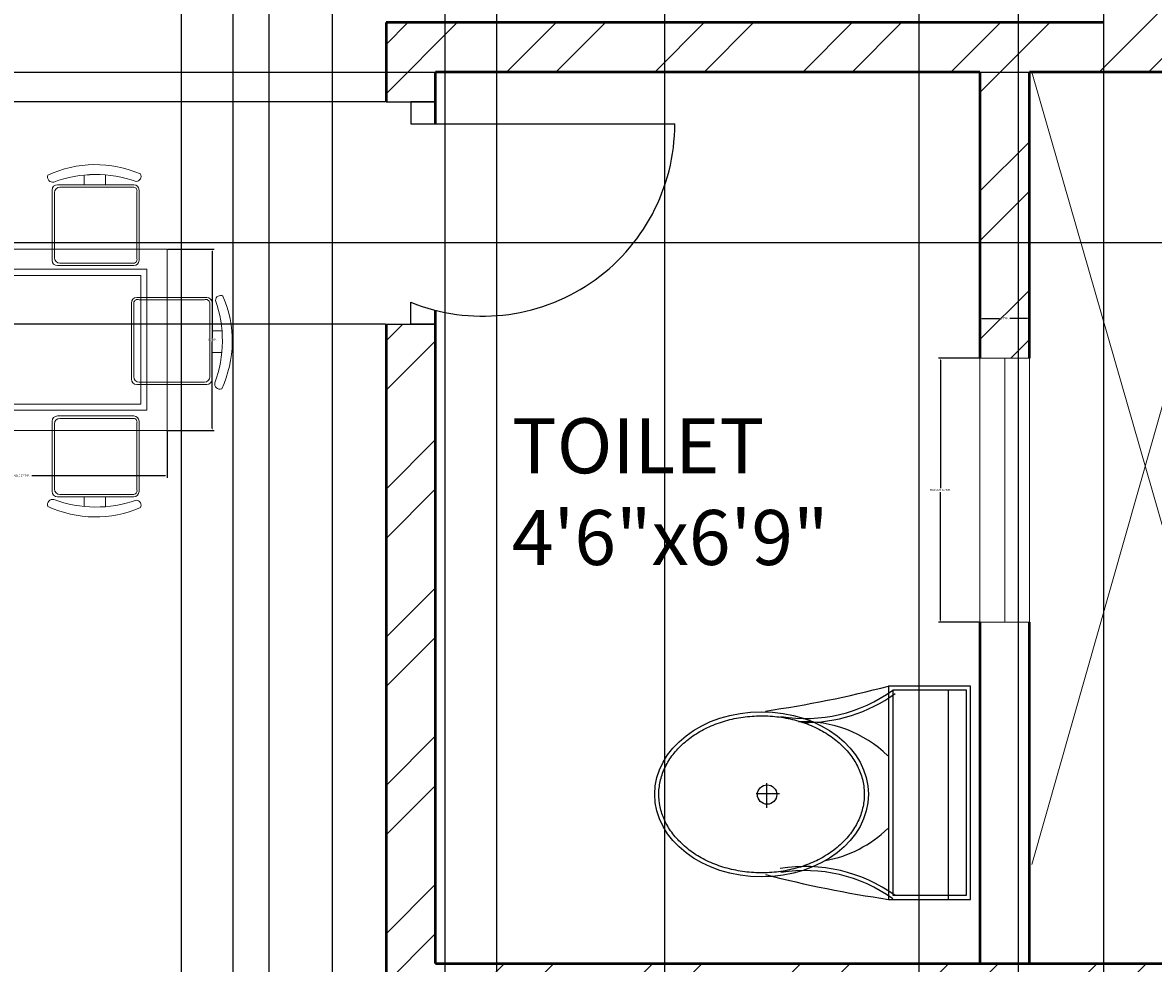
# Model space of a CAD drawing. Units: inches. Extents: x 1980 to 2738, y 1471 to 2568.
# Tile 6 of 22: x 2260 to 2363, y 1792 to 1878. Entities that reach past the tile are written whole.
import ezdxf

# ---------------------------------------------------------------- set-up
doc = ezdxf.new("R2010")
doc.units = ezdxf.units.IN
for name, color, linetype, lineweight in [('A-ANNO-DIMS', 2, 'Continuous', 18), ('A-AREA-IDEN', 7, 'Continuous', 18), ('A-DOOR', 31, 'Continuous', 25), ('A-FLOR-FIXT', 8, 'Continuous', 25), ('A-FLOR-OPEN', 8, 'Continuous', 18), ('A-FURN', 8, 'Continuous', 18), ('A-GLAZ', 141, 'Continuous', 18), ('A-WALL', 7, 'Continuous', 50)]:
    doc.layers.add(name, color=color, linetype=linetype, lineweight=lineweight)
doc.layers.add('A-WALL-PATT', color=9, linetype='Continuous', lineweight=13, true_color=0xd19cc7)
doc.styles.get("Standard").update_dxf_attribs({"font": 'arial.ttf'})
doc.dimstyles.get("Standard").update_dxf_attribs({"dimtxt": 0.18, "dimasz": 0.18, "dimexe": 0.18, "dimexo": 0.0625, "dimgap": 0.09, "dimtad": 0, "dimtih": 1, "dimtoh": 1, "dimdec": 4, "dimzin": 0, "dimdsep": 46, "dimtxsty": 'Standard', "dimcen": 0.09, "dimadec": 0, "dimazin": 0, "dimtfac": 1, "dimtdec": 4, "dimtofl": 0, "dimtmove": 0, "dimatfit": 3, "dimfxl": 1, "dimtolj": 1, "dimtzin": 0, "dimarcsym": 0})

# ---------------------------------------------------------------- blocks, each defined once
blk = doc.blocks.new('A$C31115884')
for p, q in [((283.1, 497.7), (223.4, 497.7)), ((257.5, 466.4), (257.5, 523.2)), ((0, 200), (0, 0)), ((520, 200), (0, 200)), ((520, 0), (520, 200)), ((10, 190), (10, 10)), ((510, 190), (10, 190)), ((510, 10), (510, 190)), ((510, 54.5), (0, 54.5)), ((10, 10), (510, 10)), ((0, 0), (520, 0))]:
    blk.add_line(p, q)
blk.add_circle((255.6, 496.4), 23.6)
for centre, radius, start, end in [((2777.7, -204.6), 2807, 165.4549, 171.7133), ((3237, 905), 2807, 188.2867, 194.5451), ((-294.5, 403.3), 364.7, 324.2091, 9.3499), ((-294.5, 403.3), 374.7, 324.2091, 9.3499), ((805.8, 403.3), 364.7, 170.6501, 215.7909), ((139.5, 406.2), 293.5, 315.8436, 2.6563), ((805.8, 403.3), 374.7, 179.2036, 215.7909), ((383.6, 406.2), 293.5, 190.2774, 224.1564)]:
    blk.add_arc(centre, radius, start, end)
blk.add_ellipse((256.2, 509.9), major_axis=(0, -260.7), ratio=0.772727)
blk.add_open_spline([(256.2, 259.2), (263.1, 259.2), (270, 259.7), (287.8, 262.3), (298.7, 265.1), (319.9, 273.1), (330.2, 278.4), (350.1, 291.1), (359.7, 298.7), (377.7, 315.9), (386.2, 325.5), (401.7, 346.6), (408.8, 358.1), (421.3, 382.5), (426.8, 395.5), (435.9, 422.4), (439.5, 436.4), (444.8, 465.1), (446.5, 479.7), (447.9, 509.2), (447.6, 524), (445, 553.3), (442.7, 567.8), (436.3, 596), (432.1, 609.7), (421.9, 636), (416, 648.6), (402.5, 672.1), (395, 683), (378.6, 703), (369.8, 712.1), (351.1, 728), (341.3, 734.8), (320.9, 746.2), (310.4, 750.7), (288.9, 757.3), (278, 759.4), (256, 761), (245, 760.6), (223.1, 757.2), (212.3, 754.3), (191.1, 746.1), (180.8, 740.7), (160.9, 727.8), (151.4, 720.1), (133.5, 702.7), (125.1, 693), (109.6, 671.7), (102.6, 660.2), (90.2, 635.7), (84.9, 622.7), (76, 595.6), (72.4, 581.6), (67.2, 552.9), (65.6, 538.2), (64.4, 508.8), (64.8, 494), (67.5, 464.7), (69.9, 450.2), (76.6, 422), (80.8, 408.3), (91.1, 382.2), (97.2, 369.7), (110.8, 346.3), (118.4, 335.4), (134.8, 315.6), (143.7, 306.7), (162.4, 290.9), (172.3, 284.2), (192.8, 273), (203.3, 268.6), (224.8, 262.2), (235.8, 260.2), (249.9, 259.3), (253, 259.2), (256.2, 259.2)], degree=3, knots=[0, 0, 0, 0, 0.110105, 0.110105, 0.285049, 0.285049, 0.459994, 0.459994, 0.634938, 0.634938, 0.809882, 0.809882, 0.984827, 0.984827, 1.159771, 1.159771, 1.334715, 1.334715, 1.50966, 1.50966, 1.684604, 1.684604, 1.859549, 1.859549, 2.034493, 2.034493, 2.209437, 2.209437, 2.384382, 2.384382, 2.559326, 2.559326, 2.73427, 2.73427, 2.909215, 2.909215, 3.084159, 3.084159, 3.259103, 3.259103, 3.434048, 3.434048, 3.608992, 3.608992, 3.783936, 3.783936, 3.958881, 3.958881, 4.133825, 4.133825, 4.30877, 4.30877, 4.483714, 4.483714, 4.658658, 4.658658, 4.833603, 4.833603, 5.008547, 5.008547, 5.183491, 5.183491, 5.358436, 5.358436, 5.53338, 5.53338, 5.708324, 5.708324, 5.883269, 5.883269, 6.058213, 6.058213, 6.233158, 6.233158, 6.283185, 6.283185, 6.283185, 6.283185])
blk = doc.blocks.new('TABLE-DINING-RECT')
for points in [[(0, 16.47), (27.45, 16.47), (27.45, 0), (0, 0)], [(0, 16.47), (27.45, 16.47), (27.45, 0), (0, 0)], [(1.83, 14.64), (25.62, 14.64), (25.62, 1.83), (1.83, 1.83)], [(1.83, 14.64), (25.62, 14.64), (25.62, 1.83), (1.83, 1.83)], [(2.38, 14.09), (25.07, 14.09), (25.07, 2.38), (2.38, 2.38)], [(2.38, 14.09), (25.07, 14.09), (25.07, 2.38), (2.38, 2.38)]]:
    blk.add_lwpolyline(points, close=True)
blk = doc.blocks.new('WIN-24IN-PARTITION')
for p, q in [((0, 24), (4.5, 24)), ((0, 24), (0, 0)), ((4.5, 24), (2.25, 24)), ((2.25, 24), (2.25, 0)), ((4.5, 24), (4.5, 0)), ((2.25, 0), (0, 0)), ((0, 0), (4.5, 0))]:
    blk.add_line(p, q)
blk = doc.blocks.new('SHAFT-OPENING-MARK')
for p, q in [((20.51, 72), (0, 0)), ((0, 72), (20.71, 0.06))]:
    blk.add_line(p, q)
blk = doc.blocks.new('*D21')
at = {"layer": 'A-ANNO-DIMS', "color": 0, "lineweight": -2, "transparency": 16777216}
for p, q in [((2245.93, 1840.58), (2245.93, 1836.35)), ((2273.38, 1840.58), (2273.38, 1836.35)), ((2246.11, 1836.53), (2258.22, 1836.53)), ((2273.2, 1836.53), (2261.09, 1836.53))]:
    blk.add_line(p, q, dxfattribs=at)
at = {"layer": 'A-ANNO-DIMS', "color": 0, "transparency": 16777216}
for points in [[(2246.11, 1836.56), (2246.11, 1836.5), (2245.93, 1836.53)], [(2273.2, 1836.56), (2273.2, 1836.5), (2273.38, 1836.53)]]:
    blk.add_solid(points, dxfattribs=at)
at = {"layer": 'Defpoints', "color": 0, "transparency": 16777216}
for p in [(2245.93, 1840.64), (2273.38, 1840.64), (2273.38, 1836.53)]:
    blk.add_point(p, dxfattribs=at)
at = {"layer": 'A-ANNO-DIMS', "color": 0, "transparency": 16777216, "insert": (2259.65, 1836.53), "char_height": 0.18, "attachment_point": 5}
blk.add_mtext('\\A1;DINING TABLE 27 TYP.', dxfattribs=at)
blk = doc.blocks.new('*D22')
at = {"layer": 'A-ANNO-DIMS', "color": 0, "lineweight": -2, "transparency": 16777216}
for p, q in [((2273.44, 1857.11), (2277.67, 1857.11)), ((2277.49, 1856.93), (2277.49, 1849.06)), ((2277.49, 1840.82), (2277.49, 1848.7)), ((2273.44, 1840.64), (2277.67, 1840.64))]:
    blk.add_line(p, q, dxfattribs=at)
at = {"layer": 'A-ANNO-DIMS', "color": 0, "transparency": 16777216}
for points in [[(2277.46, 1856.93), (2277.52, 1856.93), (2277.49, 1857.11)], [(2277.46, 1840.82), (2277.52, 1840.82), (2277.49, 1840.64)]]:
    blk.add_solid(points, dxfattribs=at)
at = {"layer": 'Defpoints', "color": 0, "transparency": 16777216}
for p in [(2273.38, 1857.11), (2277.49, 1857.11), (2273.38, 1840.64)]:
    blk.add_point(p, dxfattribs=at)
at = {"layer": 'A-ANNO-DIMS', "color": 0, "transparency": 16777216, "insert": (2277.49, 1848.88), "char_height": 0.18, "attachment_point": 5}
blk.add_mtext('\\A1;16 TYP.', dxfattribs=at)
blk = doc.blocks.new('*D25')
at = {"layer": 'A-ANNO-DIMS', "color": 0, "lineweight": -2, "transparency": 16777216}
for p, q in [((2347.25, 1847.22), (2343.53, 1847.22)), ((2343.71, 1847.04), (2343.71, 1835.4)), ((2343.71, 1823.4), (2343.71, 1835.04)), ((2347.25, 1823.22), (2343.53, 1823.22))]:
    blk.add_line(p, q, dxfattribs=at)
at = {"layer": 'A-ANNO-DIMS', "color": 0, "transparency": 16777216}
for points in [[(2343.68, 1847.04), (2343.74, 1847.04), (2343.71, 1847.22)], [(2343.68, 1823.4), (2343.74, 1823.4), (2343.71, 1823.22)]]:
    blk.add_solid(points, dxfattribs=at)
at = {"layer": 'Defpoints', "color": 0, "transparency": 16777216}
for p in [(2343.71, 1847.22), (2347.31, 1847.22), (2347.31, 1823.22)]:
    blk.add_point(p, dxfattribs=at)
at = {"layer": 'A-ANNO-DIMS', "color": 0, "transparency": 16777216, "insert": (2343.71, 1835.22), "char_height": 0.18, "attachment_point": 5}
blk.add_mtext('\\A1;WINDOW 24 TYP.', dxfattribs=at)
blk = doc.blocks.new('*D26')
at = {"layer": 'A-ANNO-DIMS', "color": 0, "lineweight": -2, "transparency": 16777216}
for p, q in [((2347.31, 1847.28), (2347.31, 1851)), ((2347.49, 1850.82), (2349.1, 1850.82)), ((2351.63, 1850.82), (2350.02, 1850.82)), ((2351.81, 1847.28), (2351.81, 1851))]:
    blk.add_line(p, q, dxfattribs=at)
at = {"layer": 'A-ANNO-DIMS', "color": 0, "transparency": 16777216}
for points in [[(2347.49, 1850.85), (2347.49, 1850.79), (2347.31, 1850.82)], [(2351.63, 1850.85), (2351.63, 1850.79), (2351.81, 1850.82)]]:
    blk.add_solid(points, dxfattribs=at)
at = {"layer": 'Defpoints', "color": 0, "transparency": 16777216}
for p in [(2351.81, 1850.82), (2347.31, 1847.22), (2351.81, 1847.22)]:
    blk.add_point(p, dxfattribs=at)
at = {"layer": 'A-ANNO-DIMS', "color": 0, "transparency": 16777216, "insert": (2349.56, 1850.82), "char_height": 0.18, "attachment_point": 5}
blk.add_mtext('\\A1;5 TYP.', dxfattribs=at)
blk = doc.blocks.new('*D40')
at = {"layer": 'A-ANNO-DIMS', "color": 0, "lineweight": -2, "transparency": 16777216}
for p, q in [((2218.65, 2053.14), (2218.65, 1533.71)), ((2298.65, 2053.14), (2298.65, 1533.71)), ((2218.83, 1533.89), (2258.43, 1533.89)), ((2298.47, 1533.89), (2258.87, 1533.89))]:
    blk.add_line(p, q, dxfattribs=at)
at = {"layer": 'A-ANNO-DIMS', "color": 0, "transparency": 16777216}
for points in [[(2218.83, 1533.92), (2218.83, 1533.86), (2218.65, 1533.89)], [(2298.47, 1533.92), (2298.47, 1533.86), (2298.65, 1533.89)]]:
    blk.add_solid(points, dxfattribs=at)
at = {"layer": 'Defpoints', "color": 0, "transparency": 16777216}
for p in [(2218.65, 2053.21), (2298.65, 2053.21), (2298.65, 1533.89)]:
    blk.add_point(p, dxfattribs=at)
at = {"layer": 'A-ANNO-DIMS', "color": 0, "transparency": 16777216, "insert": (2258.65, 1533.89), "char_height": 0.18, "attachment_point": 5}
blk.add_mtext('\\A1;80', dxfattribs=at)
blk = doc.blocks.new('*D41')
at = {"layer": 'A-ANNO-DIMS', "color": 0, "lineweight": -2, "transparency": 16777216}
for p, q in [((2298.65, 2095.14), (2298.65, 1533.71)), ((2515.4, 2095.14), (2515.4, 1533.71)), ((2298.83, 1533.89), (2406.56, 1533.89)), ((2515.22, 1533.89), (2407.49, 1533.89))]:
    blk.add_line(p, q, dxfattribs=at)
at = {"layer": 'A-ANNO-DIMS', "color": 0, "transparency": 16777216}
for points in [[(2298.83, 1533.92), (2298.83, 1533.86), (2298.65, 1533.89)], [(2515.22, 1533.92), (2515.22, 1533.86), (2515.4, 1533.89)]]:
    blk.add_solid(points, dxfattribs=at)
at = {"layer": 'Defpoints', "color": 0, "transparency": 16777216}
for p in [(2298.65, 2095.21), (2515.4, 2095.21), (2515.4, 1533.89)]:
    blk.add_point(p, dxfattribs=at)
at = {"layer": 'A-ANNO-DIMS', "color": 0, "transparency": 16777216, "insert": (2407.03, 1533.89), "char_height": 0.18, "attachment_point": 5}
blk.add_mtext('\\A1;216.75', dxfattribs=at)
blk = doc.blocks.new('*D45')
at = {"layer": 'A-ANNO-DIMS', "color": 0, "lineweight": -2, "transparency": 16777216}
for p, q in [((2255.99, 1694.77), (2255.99, 2507.54)), ((2256.17, 2507.36), (2267.22, 2507.36)), ((2279.21, 2507.36), (2268.15, 2507.36)), ((2279.39, 1694.77), (2279.39, 2507.54))]:
    blk.add_line(p, q, dxfattribs=at)
at = {"layer": 'A-ANNO-DIMS', "color": 0, "transparency": 16777216}
for points in [[(2256.17, 2507.39), (2256.17, 2507.33), (2255.99, 2507.36)], [(2279.21, 2507.39), (2279.21, 2507.33), (2279.39, 2507.36)]]:
    blk.add_solid(points, dxfattribs=at)
at = {"layer": 'Defpoints', "color": 0, "transparency": 16777216}
for p in [(2279.39, 2507.36), (2255.99, 1694.71), (2279.39, 1694.71)]:
    blk.add_point(p, dxfattribs=at)
at = {"layer": 'A-ANNO-DIMS', "color": 0, "transparency": 16777216, "insert": (2267.69, 2507.36), "char_height": 0.18, "attachment_point": 5}
blk.add_mtext('\\A1;23.407', dxfattribs=at)
blk = doc.blocks.new('*D50')
at = {"layer": 'A-ANNO-DIMS', "color": 0, "lineweight": -2, "transparency": 16777216}
for p, q in [((2288.43, 1708.09), (2288.43, 2507.54)), ((2288.61, 2507.36), (2314.71, 2507.36)), ((2341.6, 2507.36), (2315.5, 2507.36)), ((2341.78, 1708.09), (2341.78, 2507.54))]:
    blk.add_line(p, q, dxfattribs=at)
at = {"layer": 'A-ANNO-DIMS', "color": 0, "transparency": 16777216}
for points in [[(2288.61, 2507.39), (2288.61, 2507.33), (2288.43, 2507.36)], [(2341.6, 2507.39), (2341.6, 2507.33), (2341.78, 2507.36)]]:
    blk.add_solid(points, dxfattribs=at)
at = {"layer": 'Defpoints', "color": 0, "transparency": 16777216}
for p in [(2341.78, 2507.36), (2288.43, 1708.03), (2341.78, 1708.03)]:
    blk.add_point(p, dxfattribs=at)
at = {"layer": 'A-ANNO-DIMS', "color": 0, "transparency": 16777216, "insert": (2315.11, 2507.36), "char_height": 0.18, "attachment_point": 5}
blk.add_mtext('\\A1;53.34', dxfattribs=at)
blk = doc.blocks.new('*D51')
at = {"layer": 'A-ANNO-DIMS', "color": 0, "lineweight": -2, "transparency": 16777216}
for p, q in [((2341.78, 1708.09), (2341.78, 2507.54)), ((2341.96, 2507.36), (2349.72, 2507.36)), ((2358.4, 2507.36), (2350.63, 2507.36)), ((2358.58, 1694.77), (2358.58, 2507.54))]:
    blk.add_line(p, q, dxfattribs=at)
at = {"layer": 'A-ANNO-DIMS', "color": 0, "transparency": 16777216}
for points in [[(2341.96, 2507.39), (2341.96, 2507.33), (2341.78, 2507.36)], [(2358.4, 2507.39), (2358.4, 2507.33), (2358.58, 2507.36)]]:
    blk.add_solid(points, dxfattribs=at)
at = {"layer": 'Defpoints', "color": 0, "transparency": 16777216}
for p in [(2358.58, 2507.36), (2341.78, 1708.03), (2358.58, 1694.71)]:
    blk.add_point(p, dxfattribs=at)
at = {"layer": 'A-ANNO-DIMS', "color": 0, "transparency": 16777216, "insert": (2350.18, 2507.36), "char_height": 0.18, "attachment_point": 5}
blk.add_mtext('\\A1;16.807', dxfattribs=at)
blk = doc.blocks.new('*D53')
at = {"layer": 'A-ANNO-DIMS', "color": 0, "lineweight": -2, "transparency": 16777216}
for p, q in [((2318.63, 2002.14), (2318.63, 1533.71)), ((2350.79, 2002.14), (2350.79, 1533.71)), ((2318.81, 1533.89), (2334.25, 1533.89)), ((2350.61, 1533.89), (2335.18, 1533.89))]:
    blk.add_line(p, q, dxfattribs=at)
at = {"layer": 'A-ANNO-DIMS', "color": 0, "transparency": 16777216}
for points in [[(2318.81, 1533.92), (2318.81, 1533.86), (2318.63, 1533.89)], [(2350.61, 1533.92), (2350.61, 1533.86), (2350.79, 1533.89)]]:
    blk.add_solid(points, dxfattribs=at)
at = {"layer": 'Defpoints', "color": 0, "transparency": 16777216}
for p in [(2318.63, 2002.21), (2350.79, 2002.21), (2350.79, 1533.89)]:
    blk.add_point(p, dxfattribs=at)
at = {"layer": 'A-ANNO-DIMS', "color": 0, "transparency": 16777216, "insert": (2334.71, 1533.89), "char_height": 0.18, "attachment_point": 5}
blk.add_mtext('\\A1;32.155', dxfattribs=at)
blk = doc.blocks.new('*D61')
at = {"layer": 'A-ANNO-DIMS', "color": 0, "lineweight": -2, "transparency": 16777216}
for p, q in [((2114.15, 1873.21), (2689.91, 1873.21)), ((2689.73, 1873.03), (2689.73, 1865.65)), ((2689.73, 1857.91), (2689.73, 1865.29)), ((2114.15, 1857.73), (2689.91, 1857.73))]:
    blk.add_line(p, q, dxfattribs=at)
at = {"layer": 'A-ANNO-DIMS', "color": 0, "transparency": 16777216}
for points in [[(2689.7, 1873.03), (2689.76, 1873.03), (2689.73, 1873.21)], [(2689.7, 1857.91), (2689.76, 1857.91), (2689.73, 1857.73)]]:
    blk.add_solid(points, dxfattribs=at)
at = {"layer": 'Defpoints', "color": 0, "transparency": 16777216}
for p in [(2114.08, 1873.21), (2689.73, 1873.21), (2114.08, 1857.73)]:
    blk.add_point(p, dxfattribs=at)
at = {"layer": 'A-ANNO-DIMS', "color": 0, "transparency": 16777216, "insert": (2689.73, 1865.47), "char_height": 0.18, "attachment_point": 5}
blk.add_mtext('\\A1;15.48', dxfattribs=at)
blk = doc.blocks.new('*D64')
at = {"layer": 'A-ANNO-DIMS', "color": 0, "lineweight": -2, "transparency": 16777216}
for p, q in [((2303.33, 2002.14), (2303.33, 1533.71)), ((2318.63, 2002.14), (2318.63, 1533.71)), ((2303.51, 1533.89), (2310.67, 1533.89)), ((2318.45, 1533.89), (2311.3, 1533.89))]:
    blk.add_line(p, q, dxfattribs=at)
at = {"layer": 'A-ANNO-DIMS', "color": 0, "transparency": 16777216}
for points in [[(2303.51, 1533.92), (2303.51, 1533.86), (2303.33, 1533.89)], [(2318.45, 1533.92), (2318.45, 1533.86), (2318.63, 1533.89)]]:
    blk.add_solid(points, dxfattribs=at)
at = {"layer": 'Defpoints', "color": 0, "transparency": 16777216}
for p in [(2303.33, 2002.21), (2318.63, 2002.21), (2318.63, 1533.89)]:
    blk.add_point(p, dxfattribs=at)
at = {"layer": 'A-ANNO-DIMS', "color": 0, "transparency": 16777216, "insert": (2310.98, 1533.89), "char_height": 0.18, "attachment_point": 5}
blk.add_mtext('\\A1;15.3', dxfattribs=at)
blk = doc.blocks.new('*D65')
at = {"layer": 'A-ANNO-DIMS', "color": 0, "lineweight": -2, "transparency": 16777216}
for p, q in [((2293.25, 1870.5), (2036.25, 1870.5)), ((2036.43, 1870.32), (2036.43, 1860.58)), ((2036.43, 1850.47), (2036.43, 1860.21)), ((2293.25, 1850.29), (2036.25, 1850.29))]:
    blk.add_line(p, q, dxfattribs=at)
at = {"layer": 'A-ANNO-DIMS', "color": 0, "transparency": 16777216}
for points in [[(2036.4, 1870.32), (2036.46, 1870.32), (2036.43, 1870.5)], [(2036.4, 1850.47), (2036.46, 1850.47), (2036.43, 1850.29)]]:
    blk.add_solid(points, dxfattribs=at)
at = {"layer": 'Defpoints', "color": 0, "transparency": 16777216}
for p in [(2036.43, 1870.5), (2293.31, 1870.5), (2293.31, 1850.29)]:
    blk.add_point(p, dxfattribs=at)
at = {"layer": 'A-ANNO-DIMS', "color": 0, "transparency": 16777216, "insert": (2036.43, 1860.4), "char_height": 0.18, "attachment_point": 5}
blk.add_mtext('\\A1;20.204', dxfattribs=at)
blk = doc.blocks.new('*D66')
at = {"layer": 'A-ANNO-DIMS', "color": 0, "lineweight": -2, "transparency": 16777216}
for p, q in [((2274.65, 2095.14), (2274.65, 1533.71)), ((2282.65, 2095.14), (2282.65, 1533.71)), ((2274.83, 1533.89), (2278.5, 1533.89)), ((2282.47, 1533.89), (2278.8, 1533.89))]:
    blk.add_line(p, q, dxfattribs=at)
at = {"layer": 'A-ANNO-DIMS', "color": 0, "transparency": 16777216}
for points in [[(2274.83, 1533.92), (2274.83, 1533.86), (2274.65, 1533.89)], [(2282.47, 1533.92), (2282.47, 1533.86), (2282.65, 1533.89)]]:
    blk.add_solid(points, dxfattribs=at)
at = {"layer": 'Defpoints', "color": 0, "transparency": 16777216}
for p in [(2274.65, 2095.21), (2282.65, 2095.21), (2282.65, 1533.89)]:
    blk.add_point(p, dxfattribs=at)
at = {"layer": 'A-ANNO-DIMS', "color": 0, "transparency": 16777216, "insert": (2278.65, 1533.89), "char_height": 0.18, "attachment_point": 5}
blk.add_mtext('\\A1;8', dxfattribs=at)

msp = doc.modelspace()

# ---------------------------------------------------------------- hatches: boundary and pattern name
at = {"layer": 'A-WALL-PATT'}
h = msp.add_hatch(dxfattribs=at)
h.set_pattern_fill('ANSI32', color=256)
h.paths.add_polyline_path([(2257.5661, 2416.2064), (2257.5661, 2420.7064), (2250.5833, 2420.7064), (2250.5833, 2462.7064), (2246.0833, 2462.7064), (2246.0833, 2420.7064), (2237.0791, 2420.7064), (2237.0791, 2411.7064), (2246.0833, 2411.7064), (2246.0833, 2291.7064), (2242.6109, 2291.7064), (2242.6109, 2287.2064), (2246.0833, 2287.2064), (2250.5833, 2287.2064), (2250.5833, 2291.7064), (2250.5833, 2411.7064), (2257.5661, 2411.7064)])
h.paths.add_polyline_path([(2387.0396, 2416.2064), (2387.0396, 2420.7064), (2367.5833, 2420.7064), (2367.5833, 2462.7064), (2358.5833, 2462.7064), (2358.5833, 2420.7064), (2329.3087, 2420.7064), (2329.3087, 2411.7064), (2358.5833, 2411.7064), (2358.5833, 2321.7275), (2358.5833, 2309.7064), (2347.3089, 2309.7064), (2293.3089, 2309.7064), (2293.3089, 2259.0771), (2297.8089, 2259.0771), (2297.8089, 2305.2064), (2347.3089, 2305.2064), (2347.3089, 2284.7412), (2351.8089, 2284.7412), (2351.8089, 2305.2064), (2372.3188, 2305.2064), (2372.3761, 2284.3899), (2377.0295, 2284.3899), (2377.0295, 2299.3058), (2377.0295, 2305.2064), (2426.5295, 2305.2064), (2426.5295, 2257.5573), (2431.0295, 2257.5573), (2431.0295, 2309.7064), (2377.0295, 2309.7064), (2367.5833, 2309.7064), (2367.5833, 2321.7275), (2367.5833, 2411.7064), (2387.0396, 2411.7064)])
h.paths.add_polyline_path([(2448.5267, 2416.2064), (2448.5267, 2420.7064), (2423.0396, 2420.7064), (2423.0396, 2411.7064), (2448.5267, 2411.7064)])
h.paths.add_polyline_path([(2130.9128, 2416.2064), (2130.9128, 2420.7064), (2105.0833, 2420.7064), (2105.0833, 2386.6942), (2114.0833, 2386.6942), (2114.0833, 2411.7064), (2130.9128, 2411.7064)])
h.paths.add_polyline_path([(2212.9478, 2420.7064), (2190.9128, 2420.7064), (2190.9128, 2411.7064), (2212.9478, 2411.7064), (2212.9478, 2416.2064)])
h.paths.add_polyline_path([(2114.0833, 2326.6942), (2105.0833, 2326.6942), (2105.0833, 2291.7064), (2081.0833, 2291.7064), (2081.0833, 2287.2064), (2105.0833, 2287.2064), (2105.0833, 2276.1935), (2114.0833, 2276.1935), (2114.0833, 2287.2064), (2166.3825, 2287.2064), (2166.3825, 2289.4564), (2166.3825, 2291.7064), (2114.0833, 2291.7064)])
h.paths.add_polyline_path([(2114.0833, 2252.1935), (2105.0833, 2252.1935), (2105.0833, 2233.2064), (2081.0833, 2233.2064), (2081.0833, 2228.7064), (2105.0833, 2228.7064), (2105.0833, 2213.4478), (2114.0833, 2213.4478), (2114.0833, 2228.7064), (2195.0833, 2228.7064), (2199.5833, 2228.7064), (2208.4455, 2228.7064), (2208.4455, 2230.9564), (2208.4455, 2233.2064), (2199.5833, 2233.2064), (2199.5833, 2287.2064), (2206.8904, 2287.2064), (2206.8904, 2289.4564), (2206.8904, 2291.7064), (2189.446, 2291.7064), (2189.446, 2289.4564), (2189.446, 2287.2064), (2195.0833, 2287.2064), (2195.0833, 2233.2064), (2114.0833, 2233.2064)])
h.paths.add_polyline_path([(2114.0833, 2153.4478), (2109.5833, 2153.4478), (2105.0833, 2153.4478), (2105.0833, 2135.2374), (2114.0833, 2135.2374)], flags=17)
h.paths.add_polyline_path([(2135.9619, 2095.4081), (2140.1805, 2095.4081), (2140.1805, 2104.2064), (2114.0833, 2104.2064), (2114.0833, 2110.3997), (2109.5833, 2110.3997), (2105.0833, 2110.3997), (2105.0833, 2104.2064), (2081.0833, 2104.2064), (2081.0833, 2099.7064), (2105.0833, 2099.7064), (2127.5416, 2099.8532), (2127.5416, 2056.9393), (2136.2133, 2056.9393)], flags=17)
h.paths.add_polyline_path([(2255.4895, 2104.2064), (2250.5833, 2104.2064), (2250.5833, 2233.2064), (2246.0833, 2233.2064), (2242.4941, 2233.2064), (2242.4941, 2228.7064), (2246.0833, 2228.7064), (2246.0833, 2104.2064), (2163.6825, 2104.2064), (2163.6825, 2099.8072), (2163.6825, 2095.4081), (2191.4325, 2095.4081), (2191.4325, 2011.2064), (2186.0833, 2011.2064), (2136.5143, 2010.8824), (2136.3702, 2032.9403), (2131.9559, 2032.9115), (2127.5416, 2032.8826), (2127.5416, 2006.7064), (2105.0833, 2006.7064), (2081.0833, 2006.7064), (2081.0833, 2002.2064), (2105.0833, 2002.2064), (2105.0833, 1995.9329), (2114.0833, 1995.9329), (2114.0833, 2002.2064), (2246.0833, 2002.2064), (2246.0833, 1877.7064), (2242.1358, 1877.7064), (2242.1358, 1873.2064), (2250.5833, 1873.2064), (2250.5833, 2002.2064), (2255.3335, 2002.2064), (2255.3335, 2011.2064), (2195.9325, 2011.2064), (2195.9325, 2095.2064), (2255.4895, 2095.2064), (2255.4895, 2099.5471)])
h.paths.add_polyline_path([(2199.5833, 1873.2064), (2209.827, 1873.2064), (2209.827, 1875.4564), (2209.827, 1877.7064), (2114.0833, 1877.7064), (2114.0833, 1890.0968), (2105.0833, 1890.0968), (2105.0833, 1877.7064), (2081.0833, 1877.7064), (2081.0833, 1873.2064), (2105.0833, 1873.2064), (2105.0833, 1857.7279), (2114.0833, 1857.7279), (2114.0833, 1873.2064), (2195.0833, 1873.2064), (2195.0833, 1819.2064), (2190.298, 1819.2064), (2190.298, 1814.7064), (2209.8976, 1814.7064), (2209.8976, 1816.9564), (2209.8976, 1819.2064), (2199.5833, 1819.2064)])
h.paths.add_polyline_path([(2114.0833, 1814.7064), (2166.2538, 1814.7064), (2166.2538, 1816.9564), (2166.2538, 1819.2064), (2114.0833, 1819.2064), (2114.0833, 1833.7279), (2109.5833, 1833.7279), (2105.0833, 1833.7279), (2105.0833, 1819.2064), (2081.0833, 1819.2064), (2081.0833, 1814.7064), (2105.0833, 1814.7064), (2105.0833, 1782.5516), (2114.0833, 1782.5516)])
h.paths.add_polyline_path([(2114.0833, 1722.5516), (2109.5833, 1722.5516), (2105.0833, 1722.5516), (2105.0833, 1685.7064), (2124.5104, 1685.7064), (2124.5104, 1690.2064), (2124.5104, 1694.7064), (2114.0833, 1694.7064)])
h.paths.add_polyline_path([(2218.8787, 1694.7064), (2184.5104, 1694.7064), (2184.5104, 1685.7064), (2218.8787, 1685.7064), (2218.8787, 1690.2064)])
h.paths.add_polyline_path([(2250.5833, 1819.2064), (2242.6431, 1819.2064), (2242.6431, 1816.9564), (2242.6431, 1814.7064), (2246.0833, 1814.7064), (2246.0833, 1694.7064), (2240.4035, 1694.7064), (2240.4035, 1690.2064), (2240.4035, 1685.7064), (2246.0833, 1685.7064), (2246.0833, 1643.7064), (2250.5833, 1643.7064), (2250.5833, 1685.7064), (2255.9859, 1685.7064), (2255.9859, 1690.2064), (2255.9859, 1694.7064), (2250.5833, 1694.7064)])
h.paths.add_polyline_path([(2297.4764, 1694.7064), (2279.3934, 1694.7064), (2279.3934, 1690.2064), (2279.3934, 1685.7064), (2297.4764, 1685.7064), (2297.4764, 1690.2064)])
h.paths.add_polyline_path([(2377.1596, 1694.7064), (2367.5833, 1694.7064), (2367.5833, 1787.7064), (2431.0295, 1787.7064), (2431.0295, 1792.2064), (2431.0295, 1849.4149), (2428.7795, 1849.4149), (2426.5295, 1849.4149), (2426.5295, 1792.2064), (2421.5833, 1792.2064), (2367.5833, 1792.2064), (2297.8089, 1792.2064), (2297.8089, 1850.2946), (2295.5589, 1850.2946), (2293.3089, 1850.2946), (2293.3089, 1792.2064), (2293.3089, 1787.7064), (2297.8089, 1787.7064), (2358.5833, 1787.7064), (2358.5833, 1694.7064), (2333.4764, 1694.7064), (2333.4764, 1685.7064), (2358.5833, 1685.7064), (2358.5833, 1643.7064), (2367.5833, 1643.7064), (2367.5833, 1685.7064), (2377.1596, 1685.7064)])
h.paths.add_polyline_path([(2442.4912, 1694.7064), (2413.1596, 1694.7064), (2413.1596, 1685.7064), (2442.4912, 1685.7064)])
h.paths.add_polyline_path([(2480.0833, 1814.7064), (2483.4816, 1814.7064), (2483.4816, 1817.9384), (2483.4816, 1819.2064), (2475.5833, 1819.2064), (2475.5833, 1694.7064), (2470.7283, 1694.7064), (2470.7283, 1685.7064), (2475.5833, 1685.7064), (2475.5833, 1643.7064), (2480.0833, 1643.7064), (2480.0833, 1685.7064), (2486.3293, 1685.7064), (2486.3293, 1690.2064), (2486.3293, 1694.7064), (2480.0833, 1694.7064)])
h.paths.add_polyline_path([(2621.0833, 1721.7349), (2612.0833, 1721.7349), (2612.0833, 1694.7064), (2586.1453, 1694.7064), (2586.1453, 1685.7064), (2621.0833, 1685.7064)])
h.paths.add_polyline_path([(2526.1453, 1690.2064), (2526.1453, 1694.7064), (2511.584, 1694.7064), (2511.584, 1690.2064), (2511.584, 1685.7064), (2526.1453, 1685.7064)])
h.paths.add_polyline_path([(2645.0833, 1819.2064), (2621.0833, 1819.2064), (2621.0833, 1835.8527), (2616.5833, 1835.8527), (2612.0833, 1835.8527), (2612.0833, 1819.2064), (2560.2541, 1819.2064), (2560.2541, 1814.7064), (2612.0833, 1814.7064), (2612.0833, 1781.7349), (2621.0833, 1781.7349), (2621.0833, 1814.7064), (2645.0833, 1814.7064)])
h.paths.add_polyline_path([(2645.0833, 1877.7064), (2621.0833, 1877.7064), (2621.0833, 1886.4375), (2612.0833, 1886.4375), (2612.0833, 1877.7064), (2517.1032, 1877.7064), (2517.1032, 1875.4564), (2517.1032, 1873.2064), (2526.5833, 1873.2064), (2526.5833, 1819.2064), (2516.6454, 1819.2064), (2516.6454, 1816.9564), (2516.6454, 1814.7064), (2536.4445, 1814.7064), (2536.4445, 1816.9564), (2536.4445, 1819.2064), (2531.0833, 1819.2064), (2531.0833, 1873.2064), (2612.0833, 1873.2064), (2612.0833, 1859.8527), (2621.0833, 1859.8527), (2621.0833, 1873.2064), (2645.0833, 1873.2064)])
h.paths.add_polyline_path([(2645.0833, 2006.7064), (2621.0833, 2006.7064), (2588.5085, 2006.7064), (2588.5085, 2052.9125), (2579.9045, 2052.9125), (2579.9045, 2011.2064), (2519.9045, 2011.2064), (2519.9045, 2095.2064), (2553.1204, 2095.2064), (2553.1204, 2104.2064), (2480.0833, 2104.2064), (2480.0833, 2228.7064), (2484.3832, 2228.7064), (2484.3832, 2230.9564), (2484.3832, 2233.2064), (2475.5833, 2233.2064), (2475.5833, 2104.2064), (2463.1308, 2104.2064), (2463.1308, 2095.2064), (2501.2463, 2095.2064), (2510.9045, 2095.2064), (2515.4045, 2095.2064), (2515.4045, 2011.2064), (2510.9045, 2011.2064), (2501.2463, 2011.2064), (2462.5957, 2011.2064), (2462.5957, 2002.2064), (2475.5833, 2002.2064), (2475.5833, 1873.2064), (2483.6146, 1873.2064), (2483.6146, 1875.4564), (2483.6146, 1877.7064), (2480.0833, 1877.7064), (2480.0833, 2002.2064), (2612.0833, 2002.2064), (2612.0833, 1996.309), (2621.0833, 1996.309), (2621.0833, 2002.2064), (2645.0833, 2002.2064)])
h.paths.add_polyline_path([(2588.5085, 2099.7277), (2621.0833, 2099.7277), (2645.0833, 2099.7064), (2645.0833, 2104.2064), (2621.0833, 2104.2064), (2621.0833, 2109.0038), (2616.5833, 2109.0038), (2612.0833, 2109.0038), (2612.0833, 2104.2064), (2575.0621, 2104.2064), (2575.0621, 2099.7064), (2575.0621, 2095.2064), (2579.9045, 2095.2064), (2579.9045, 2076.9125), (2588.5085, 2076.9125)], flags=17)
h.paths.add_polyline_path([(2367.5833, 2002.2064), (2373.7228, 2002.2064), (2373.7228, 2006.7064), (2373.7228, 2011.2064), (2350.7889, 2011.2064), (2350.7889, 2006.7064), (2350.7889, 2002.2064), (2358.5833, 2002.2064), (2358.5833, 1877.7064), (2293.3089, 1877.7064), (2293.3089, 1870.4987), (2297.8089, 1870.4987), (2297.8089, 1873.2064), (2347.3089, 1873.2064), (2347.3089, 1847.2208), (2351.8089, 1847.2208), (2351.8089, 1873.2064), (2372.5295, 1873.2064), (2372.5295, 1847.8619), (2377.0295, 1847.8619), (2377.0295, 1873.2064), (2426.5295, 1873.2064), (2426.5295, 1868.7339), (2431.0295, 1868.7339), (2431.0295, 1877.7064), (2367.5833, 1877.7064)])
h.paths.add_polyline_path([(2531.0833, 2287.2064), (2534.2285, 2287.2064), (2534.2285, 2291.7064), (2516.7886, 2291.7064), (2516.7886, 2287.2064), (2526.5833, 2287.2064), (2526.5833, 2233.2064), (2517.9112, 2233.2064), (2517.9112, 2230.9564), (2517.9112, 2228.7064), (2526.5833, 2228.7064), (2531.0833, 2228.7064), (2612.0833, 2228.7064), (2612.0833, 2206.8504), (2621.0833, 2206.8504), (2621.0833, 2228.7064), (2645.0833, 2228.7064), (2645.0833, 2233.2064), (2621.0833, 2233.2064), (2621.0833, 2241.8536), (2616.5833, 2241.8536), (2612.0833, 2241.8536), (2612.0833, 2233.2064), (2531.0833, 2233.2064)])
h.paths.add_polyline_path([(2645.0833, 2291.7064), (2621.0833, 2291.7064), (2621.0833, 2323.0138), (2616.5833, 2323.0138), (2612.0833, 2323.0138), (2612.0833, 2291.7064), (2559.6852, 2291.7064), (2559.6852, 2289.4564), (2559.6852, 2287.2064), (2612.0833, 2287.2064), (2612.0833, 2265.8536), (2621.0833, 2265.8536), (2621.0833, 2287.2064), (2645.0833, 2287.2064)])
h.paths.add_polyline_path([(2621.0833, 2420.7064), (2582.8189, 2420.7064), (2582.8189, 2411.7064), (2612.0833, 2411.7064), (2612.0833, 2383.0138), (2621.0833, 2383.0138)])
h.paths.add_polyline_path([(2480.0833, 2411.7064), (2485.7342, 2411.7064), (2485.7342, 2416.2064), (2485.7342, 2420.7064), (2480.0833, 2420.7064), (2480.0833, 2462.7064), (2475.5833, 2462.7064), (2475.5833, 2420.7064), (2469.4083, 2420.7064), (2469.4083, 2411.7064), (2475.5833, 2411.7064), (2475.5833, 2291.7064), (2475.5833, 2287.2064), (2482.9195, 2287.2064), (2482.9195, 2289.4564), (2482.9195, 2291.7064), (2480.0833, 2291.7064)])
h.paths.add_polyline_path([(2367.5833, 2228.7064), (2431.0295, 2228.7064), (2431.0295, 2233.2064), (2431.0295, 2237.4203), (2428.7795, 2237.4203), (2426.5295, 2237.4203), (2426.5295, 2233.2064), (2377.0295, 2233.2064), (2377.0295, 2260.3837), (2372.4423, 2260.3837), (2372.517, 2233.2635), (2351.8089, 2233.2064), (2351.8089, 2260.7412), (2347.3089, 2260.7412), (2347.3089, 2233.2064), (2297.8089, 2233.2064), (2297.8089, 2236.9324), (2293.3089, 2236.9324), (2293.3089, 2228.7064), (2358.5833, 2228.7064), (2358.5833, 2104.2064), (2353.3665, 2104.2064), (2353.3665, 2095.2064), (2373.8869, 2095.2064), (2373.8869, 2099.7064), (2373.8869, 2104.2064), (2367.5833, 2104.2064)])
h.paths.add_polyline_path([(2321.2323, 2104.2064), (2303.4895, 2104.2064), (2303.4895, 2095.2064), (2321.2323, 2095.2064), (2321.2323, 2099.7064)], flags=0)
h.paths.add_polyline_path([(2415.1308, 2099.7064), (2415.1308, 2104.2064), (2404.81, 2104.2064), (2404.81, 2095.2064), (2415.1308, 2095.2064)], flags=17)
h.paths.add_polyline_path([(2318.6336, 2011.2064), (2303.3335, 2011.2064), (2303.3335, 2002.2064), (2318.6336, 2002.2064)], flags=0)
h.paths.add_polyline_path([(2414.5957, 2011.2064), (2406.2461, 2011.2064), (2406.2461, 2006.7064), (2406.2461, 2002.2064), (2414.5957, 2002.2064)], flags=17)

# ---------------------------------------------------------------- linework, layer by layer
at = {"layer": 'A-DOOR'}
for p, q in [((2293.3089, 1870.4987), (2297.8089, 1870.4987)), ((2297.8089, 1870.4987), (2295.5589, 1870.4987)), ((2295.5589, 1870.4987), (2295.5589, 1868.4987)), ((2295.5589, 1868.4987), (2319.5589, 1868.4987)), ((2295.5589, 1850.2946), (2295.5589, 1852.2946)), ((2293.3089, 1850.2946), (2297.8089, 1850.2946)), ((2297.8089, 1850.2946), (2295.5589, 1850.2946)), ((2295.5589, 1850.2946), (2295.5589, 1850.2946))]:
    msp.add_line(p, q, dxfattribs=at)
msp.add_arc((2302.0887, 1868.4987), 17.4703, 248.052221, 360, dxfattribs=at)
at = {"layer": 'A-FURN'}
for points in [[(2263.0938, 1863.217, -0.57839206), (2262.5275, 1863.8397, -0.21452438), (2270.9657, 1863.9529, -0.55201397), (2270.5693, 1863.2736, 0.1758092), (2263.0938, 1863.217)], [(2263.0939, 1863.2167, -0.57839206), (2262.5275, 1863.8394, -0.21452438), (2270.9657, 1863.9527, -0.55201397), (2270.5693, 1863.2733, 0.1758092), (2263.0939, 1863.2167)], [(2265.8486, 1862.9736), (2265.8486, 1863.8513, 0.06475861)], [(2265.8487, 1862.9733), (2265.8487, 1863.851, 0.06475861)], [(2270.3509, 1862.9736, -0.41421356), (2270.8365, 1862.4881), (2270.8365, 1856.1069, -0.41421356), (2270.3509, 1855.6214), (2263.411, 1855.6214, -0.41421356), (2262.9255, 1856.1069), (2262.9255, 1862.4881, -0.41421356), (2263.411, 1862.9736), (2270.3509, 1862.9736)], [(2270.3509, 1862.9733, -0.41421356), (2270.8365, 1862.4878), (2270.8365, 1856.1066, -0.41421356), (2270.3509, 1855.6211), (2263.411, 1855.6211, -0.41421356), (2262.9255, 1856.1066), (2262.9255, 1862.4878, -0.41421356), (2263.411, 1862.9733), (2270.3509, 1862.9733)], [(2277.4852, 1852.241, 0.41421356), (2276.9997, 1852.7265), (2270.6185, 1852.7265, 0.41421356), (2270.133, 1852.241), (2270.133, 1845.301, 0.41421356), (2270.6185, 1844.8155), (2276.9997, 1844.8155, 0.41421356), (2277.4852, 1845.301), (2277.4852, 1852.241)], [(2277.4852, 1852.2407, 0.41421356), (2276.9997, 1852.7262), (2270.6185, 1852.7262, 0.41421356), (2270.133, 1852.2407), (2270.133, 1845.3008, 0.41421356), (2270.6185, 1844.8152), (2276.9997, 1844.8152, 0.41421356), (2277.4852, 1845.3008), (2277.4852, 1852.2407)], [(2277.7852, 1852.4593, -0.17580919), (2277.7286, 1844.9839, 0.57839206), (2278.3513, 1844.4176, 0.21452438), (2278.4645, 1852.8558, 0.55201397), (2277.7852, 1852.4593, -0.06507904)], [(2277.7852, 1852.459, -0.17580919), (2277.7286, 1844.9836, 0.57839206), (2278.3513, 1844.4173, 0.21452438), (2278.4646, 1852.8555, 0.55201397), (2277.7852, 1852.459, -0.06507904)], [(2277.4852, 1847.7387), (2278.3629, 1847.7387, -0.06475861)], [(2277.4852, 1847.7384), (2278.3629, 1847.7384, -0.06475861)], [(2270.3509, 1834.6078, 0.41421356), (2270.8365, 1835.0934), (2270.8365, 1841.4745, 0.41421356), (2270.3509, 1841.96), (2263.411, 1841.96, 0.41421356), (2262.9255, 1841.4745), (2262.9255, 1835.0934, 0.41421356), (2263.411, 1834.6078), (2270.3509, 1834.6078)], [(2270.3509, 1834.6076, 0.41421356), (2270.8365, 1835.0931), (2270.8365, 1841.4742, 0.41421356), (2270.3509, 1841.9598), (2263.411, 1841.9598, 0.41421356), (2262.9255, 1841.4742), (2262.9255, 1835.0931, 0.41421356), (2263.411, 1834.6076), (2270.3509, 1834.6076)], [(2270.5693, 1834.3078, -0.17580928), (2263.0938, 1834.3644, 0.57839206), (2262.5275, 1833.7417, 0.21452438), (2270.9657, 1833.6285, 0.55201397), (2270.5693, 1834.3078, -0.06507904)], [(2270.5693, 1834.3075, -0.17580928), (2263.0939, 1834.3641, 0.57839206), (2262.5275, 1833.7414, 0.21452438), (2270.9657, 1833.6282, 0.55201397), (2270.5693, 1834.3075, -0.06507904)], [(2265.8486, 1834.6078), (2265.8486, 1833.7302, -0.06475861)], [(2265.8487, 1834.6076), (2265.8487, 1833.7299, -0.06475861)]]:
    msp.add_lwpolyline(points, format="xyb", dxfattribs=at)
for points in [[(2267.7912, 1863.8672), (2267.7912, 1862.9736)], [(2267.7913, 1863.8669), (2267.7913, 1862.9733)], [(2278.3788, 1849.6813), (2277.4852, 1849.6813)], [(2278.3788, 1849.681), (2277.4852, 1849.681)], [(2267.7912, 1833.7142), (2267.7912, 1834.6078)], [(2267.7913, 1833.7139), (2267.7913, 1834.6076)]]:
    msp.add_lwpolyline(points, dxfattribs=at)
for points in [[(2270.348, 1862.7549), (2263.6297, 1862.7549, 0.41421356), (2263.1442, 1862.2693), (2263.1442, 1856.3257, 0.41421356), (2263.6297, 1855.8401), (2270.348, 1855.8401, 0.51206948), (2270.6177, 1856.3257), (2270.6177, 1862.2693, 0.51206948)], [(2270.348, 1862.7546), (2263.6297, 1862.7546, 0.41421356), (2263.1442, 1862.269), (2263.1442, 1856.3254, 0.41421356), (2263.6297, 1855.8398), (2270.348, 1855.8398, 0.51206948), (2270.6177, 1856.3254), (2270.6177, 1862.269, 0.51206948)], [(2277.2665, 1852.238), (2277.2665, 1845.5198, -0.41421356), (2276.7809, 1845.0343), (2270.8372, 1845.0343, -0.41421356), (2270.3517, 1845.5198), (2270.3517, 1852.238, -0.51206948), (2270.8372, 1852.5078), (2276.7809, 1852.5078, -0.51206948)], [(2277.2665, 1852.2378), (2277.2665, 1845.5195, -0.41421356), (2276.7809, 1845.034), (2270.8373, 1845.034, -0.41421356), (2270.3517, 1845.5195), (2270.3517, 1852.2378, -0.51206948), (2270.8373, 1852.5075), (2276.7809, 1852.5075, -0.51206948)], [(2270.348, 1834.8266), (2263.6297, 1834.8266, -0.41421356), (2263.1442, 1835.3121), (2263.1442, 1841.2558, -0.41421356), (2263.6297, 1841.7413), (2270.348, 1841.7413, -0.51206948), (2270.6177, 1841.2558), (2270.6177, 1835.3121, -0.51206948)], [(2270.348, 1834.8263), (2263.6297, 1834.8263, -0.41421356), (2263.1442, 1835.3118), (2263.1442, 1841.2555, -0.41421356), (2263.6297, 1841.741), (2270.348, 1841.741, -0.51206948), (2270.6177, 1841.2555), (2270.6177, 1835.3118, -0.51206948)]]:
    msp.add_lwpolyline(points, format="xyb", close=True, dxfattribs=at)
at = {"layer": 'A-WALL'}
for p, q in [((2293.3089, 1877.7064), (2293.3089, 1870.4987)), ((2358.5833, 1877.7064), (2293.3089, 1877.7064)), ((2347.3089, 1873.2064), (2297.8089, 1873.2064)), ((2297.8089, 1868.4987), (2297.8089, 1873.2064)), ((2347.3089, 1873.2064), (2347.3089, 1847.2208)), ((2372.5295, 1873.2064), (2351.8089, 1873.2064)), ((2351.8089, 1847.2208), (2351.8089, 1873.2064)), ((2297.8089, 1792.2064), (2297.8089, 1851.5607)), ((2293.3089, 1850.2946), (2293.3089, 1792.2064)), ((2347.3089, 1823.2208), (2347.3089, 1792.2064)), ((2351.8089, 1792.2064), (2351.8089, 1823.2208)), ((2293.3089, 1792.2064), (2293.3089, 1792.2064)), ((2293.3089, 1792.2064), (2293.3089, 1787.7064)), ((2297.8089, 1792.2064), (2367.5833, 1792.2064)), ((2347.3089, 1792.2064), (2351.8089, 1792.2064))]:
    msp.add_line(p, q, dxfattribs=at)

# ---------------------------------------------------------------- block references
at = {"layer": 'A-FLOR-FIXT', "xscale": 0.0372717239612423, "yscale": 0.0372717239612423, "zscale": 0.0372717239612423, "rotation": 89.99999999999999}
msp.add_blockref('A$C31115884', (2346.4544, 1798.0229), dxfattribs=at)
at = {"layer": 'A-FLOR-OPEN'}
msp.add_blockref('SHAFT-OPENING-MARK', (2352.0197, 1801.206), dxfattribs=at)
at = {"layer": 'A-FURN'}
msp.add_blockref('TABLE-DINING-RECT', (2245.9301, 1840.645), dxfattribs=at)
at = {"layer": 'A-GLAZ'}
msp.add_blockref('WIN-24IN-PARTITION', (2347.3094, 1823.2209), dxfattribs=at)

# ---------------------------------------------------------------- texts
at = {"layer": 'A-AREA-IDEN', "insert": (2304.7421, 1841.7475), "char_height": 5, "attachment_point": 1}
msp.add_mtext_dynamic_manual_height_columns('TOILET\\P4\'6"x6\'9"', width=55.958855, gutter_width=12.5, heights=[0], dxfattribs=at)

# ---------------------------------------------------------------- dimensions: what is measured, and where the dimension line sits
at = {"layer": 'A-ANNO-DIMS'}
for base, p1, p2, override, picture, middle in [((2279.39337, 2507.35642), (2255.98588, 1694.70642), (2279.39337, 1694.70642), {"dimdec": 3, "dimlfac": 1, "dimrnd": 0, "dimzin": 0, "dimdsep": 46, "dimlunit": 2}, '*D45', (2267.68962, 2507.35642)), ((2341.776, 2507.3564), (2288.4349, 1708.0291), (2341.776, 1708.0291), {"dimdec": 2, "dimlfac": 1, "dimrnd": 0, "dimzin": 0, "dimdsep": 46, "dimlunit": 2}, '*D50', (2315.1054, 2507.3564)), ((2358.5833, 2507.3564), (2341.776, 1708.0291), (2358.5833, 1694.7064), {"dimdec": 3, "dimlfac": 1, "dimrnd": 0, "dimzin": 0, "dimdsep": 46, "dimlunit": 2}, '*D51', (2350.1796, 2507.3564)), ((2282.6516, 1533.8857), (2274.6516, 2095.2064), (2282.6516, 2095.2064), {"dimdec": 0, "dimlfac": 1, "dimrnd": 0, "dimzin": 0, "dimdsep": 46, "dimlunit": 2}, '*D66', (2278.6516, 1533.8857)), ((2515.4045, 1533.8857), (2298.6516, 2095.2064), (2515.4045, 2095.2064), {"dimdec": 2, "dimlfac": 1, "dimrnd": 0, "dimzin": 0, "dimdsep": 46, "dimlunit": 2}, '*D41', (2407.0281, 1533.8857)), ((2298.6516, 1533.8857), (2218.6516, 2053.2064), (2298.6516, 2053.2064), {"dimdec": 0, "dimlfac": 1, "dimrnd": 0, "dimzin": 0, "dimdsep": 46, "dimlunit": 2}, '*D40', (2258.6516, 1533.8857)), ((2318.6336, 1533.8857), (2303.3335, 2002.2064), (2318.6336, 2002.2064), {"dimdec": 1, "dimlfac": 1, "dimrnd": 0, "dimzin": 0, "dimdsep": 46, "dimlunit": 2}, '*D64', (2310.9835, 1533.8857)), ((2350.7889, 1533.8857), (2318.6336, 2002.2064), (2350.7889, 2002.2064), {"dimdec": 3, "dimlfac": 1, "dimrnd": 0, "dimzin": 0, "dimdsep": 46, "dimlunit": 2}, '*D53', (2334.7112, 1533.8857))]:
    dim = msp.add_linear_dim(base=base, p1=p1, p2=p2, dimstyle='Standard', override=override, dxfattribs=at)
    dim.commit()
    dim.dimension.update_dxf_attribs({"geometry": picture, "text_midpoint": middle})
for base, p1, p2, override, picture, middle in [((2689.7333, 1873.2064), (2114.0833, 1857.7279), (2114.0833, 1873.2064), {"dimdec": 2, "dimlfac": 1, "dimrnd": 0, "dimzin": 0, "dimdsep": 46, "dimlunit": 2}, '*D61', (2689.7333, 1865.4672)), ((2036.4333, 1870.4987), (2293.3089, 1850.2946), (2293.3089, 1870.4987), {"dimdec": 3, "dimlfac": 1, "dimrnd": 0, "dimzin": 0, "dimdsep": 46, "dimlunit": 2}, '*D65', (2036.4333, 1860.3966))]:
    dim = msp.add_linear_dim(base=base, p1=p1, p2=p2, angle=90, dimstyle='Standard', override=override, dxfattribs=at)
    dim.commit()
    dim.dimension.update_dxf_attribs({"geometry": picture, "text_midpoint": middle})
for base, p1, p2, text, picture, middle in [((2277.4929, 1857.1126), (2273.376, 1840.6449), (2273.376, 1857.1126), '<> TYP.', '*D22', (2277.4929, 1848.8788)), ((2343.7089, 1847.2208), (2347.3089, 1823.2208), (2347.3089, 1847.2208), 'WINDOW <> TYP.', '*D25', (2343.7089, 1835.2208))]:
    dim = msp.add_linear_dim(base=base, p1=p1, p2=p2, angle=90, text=text, dimstyle='Standard', override={"dimdec": 0, "dimlfac": 1, "dimrnd": 0, "dimzin": 0, "dimdsep": 46, "dimlunit": 2}, dxfattribs=at)
    dim.commit()
    dim.dimension.update_dxf_attribs({"geometry": picture, "text_midpoint": middle})
for base, p1, p2, text, picture, middle in [((2351.8089381702, 1850.8207722201), (2347.3089381702, 1847.2207722201), (2351.8089381702, 1847.2207722201), '<> TYP.', '*D26', (2349.5589381702, 1850.8207722201)), ((2273.376, 1836.528), (2245.9303, 1840.6449), (2273.376, 1840.6449), 'DINING TABLE <> TYP.', '*D21', (2259.6532, 1836.528))]:
    dim = msp.add_linear_dim(base=base, p1=p1, p2=p2, text=text, dimstyle='Standard', override={"dimdec": 0, "dimlfac": 1, "dimrnd": 0, "dimzin": 0, "dimdsep": 46, "dimlunit": 2}, dxfattribs=at)
    dim.commit()
    dim.dimension.update_dxf_attribs({"geometry": picture, "text_midpoint": middle})

doc.saveas('drawing.dxf')
